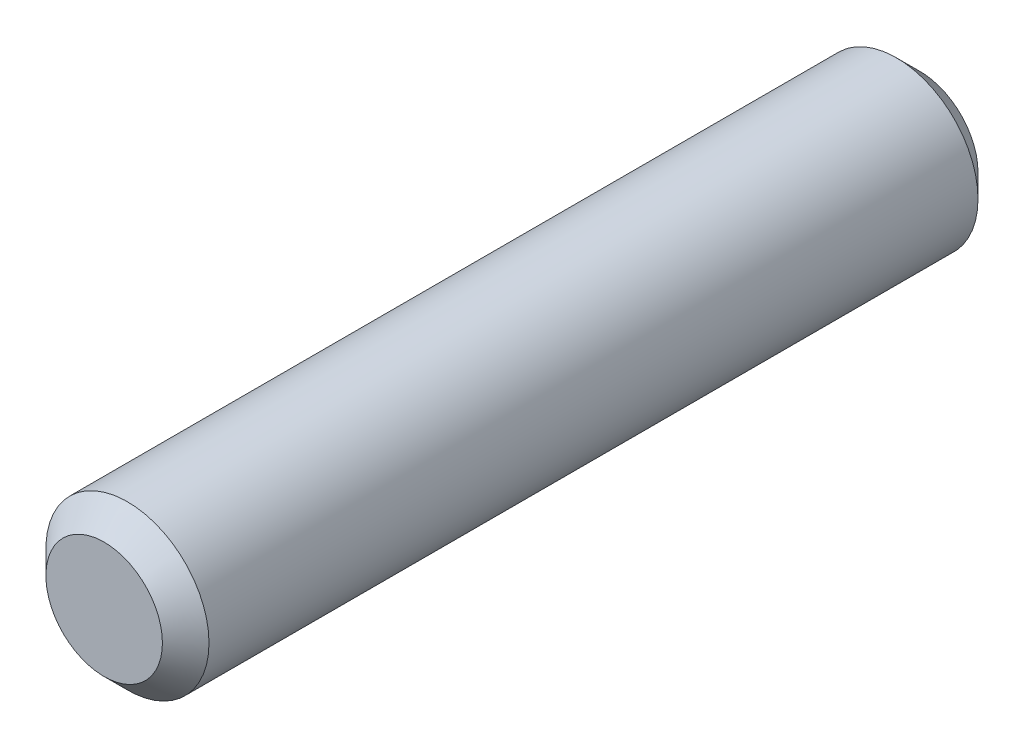
from build123d import *

# Parameters (mm, degrees)
PIN_PROFILE_14_R        = 7
PIN_BODY_14X70_DEPTH    = 35
END_CHAMFER_2X45_A_SIZE = 2
END_CHAMFER_2X45_B_SIZE = 2


with BuildPart() as part:
    # Pin Profile Ø14 → Pin Body Ø14x70 (new, symmetric)
    with BuildSketch(Plane.XY):
        Circle(PIN_PROFILE_14_R)
    extrude(amount=PIN_BODY_14X70_DEPTH, both=True)

    # End Chamfer 2x45 A
    end_chamfer_2x45_a_edges = [part.edges().sort_by_distance(p)[0] for p in [
        (-7, 0, 35),
    ]]
    chamfer(end_chamfer_2x45_a_edges, length=END_CHAMFER_2X45_A_SIZE)

    # End Chamfer 2x45 B
    end_chamfer_2x45_b_edges = [part.edges().sort_by_distance(p)[0] for p in [
        (-7, 0, -35),
    ]]
    chamfer(end_chamfer_2x45_b_edges, length=END_CHAMFER_2X45_B_SIZE)


solid = part.part
